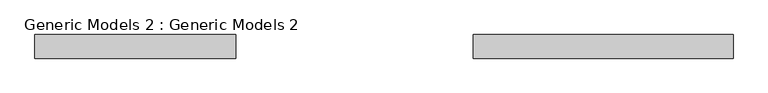
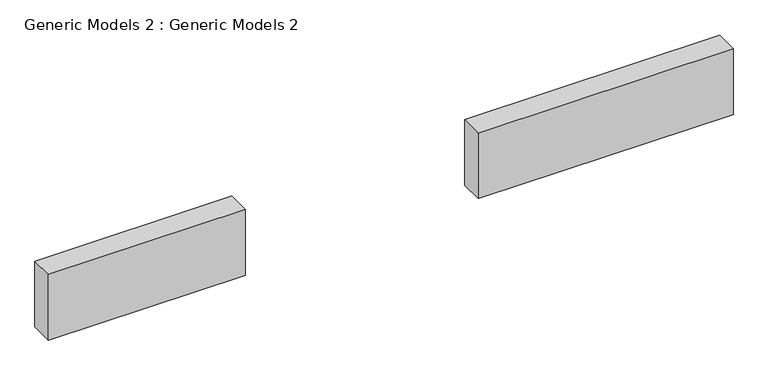
"""IFC4 building model written with IfcOpenShell, lengths in millimetres: proxy geometry, Generic Models 2 : Generic Models 2."""

from ifc_helpers import new_model, si_unit, frame, origin, place, context, project, spatial, polyline, outline, extrude, source, transform, mapped, element, save


def generic_models_2_generic_models_2_e56ad787(model_context):
    return source(origin(), model_context, "Body", "SweptSolid", [
        extrude(outline(polyline([(2960.0958131, -6563.0109248), (-392.7041869, -6563.0109248), (-392.7041869, -6258.2109248), (2960.0958131, -6258.2109248), (2960.0958131, -6563.0109248)])), frame((0.0, 0.0, 374.2241992), z_axis=(0.0, 0.0, 1.0), x_axis=(1.0, 0.0, 0.0)), (0.0, 0.0, 1.0), 914.4),
        extrude(outline(polyline([(-3456.2407788, -6563.0109248), (-6047.0407788, -6563.0109248), (-6047.0407788, -6258.2109248), (-3456.2407788, -6258.2109248), (-3456.2407788, -6563.0109248)])), frame((0.0, 0.0, 382.320447), z_axis=(0.0, 0.0, 1.0), x_axis=(1.0, 0.0, 0.0)), (0.0, 0.0, 1.0), 914.4),
    ])


if __name__ == "__main__":
    model = new_model("IFC4")
    model_context = context("Model", 3, world=origin())
    ifc_project = project(units=[si_unit("LENGTHUNIT", "METRE", prefix="MILLI")], contexts=[model_context])
    site = spatial("IfcSite", under=ifc_project)
    building = spatial("IfcBuilding", under=site)
    placement = place(None, origin())
    generic_models_2_generic_models_2_shape = generic_models_2_generic_models_2_e56ad787(model_context)
    element("IfcBuildingElementProxy", 1, Name="Generic Models 2 : Generic Models 2", ObjectType="Generic Models 2 : Generic Models 2", at=placement, inside=building, context=model_context, shape_type="MappedRepresentation", body=[
        mapped(generic_models_2_generic_models_2_shape, transform((0.0, 0.0, 0.0), x_axis=(1.0, 0.0, 0.0), y_axis=(0.0, 1.0, 0.0), z_axis=(0.0, 0.0, 1.0))),
    ])
    save(model, "model.ifc")

# Revit data of these elements
# Element 1 (IfcBuildingElementProxy, "Generic Models 2 : Generic Models 2")
#   Materials on its faces: "Laminate, Ivory, Matte"
# Materials
#   "Laminate, Ivory, Matte": class "Plastic", colour RGB 247 247 239, transparency 0, Description = "Plastic Laminate - Ivory, Matte", Cost = 0
